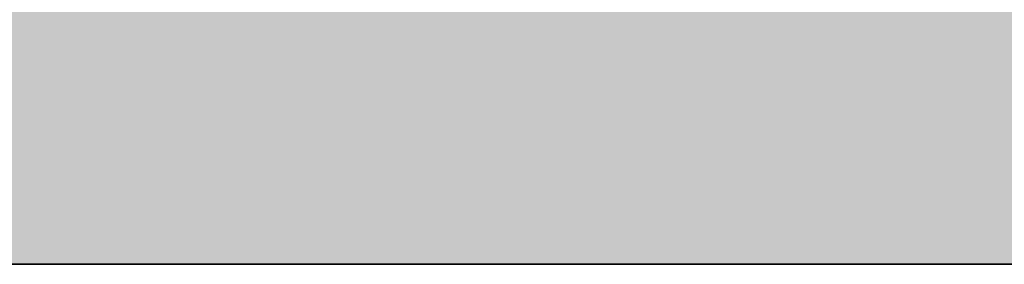
# Model space of a CAD drawing. Units: inches. Extents: x 2083 to 3317, y 1141 to 2115.
# Tile 147 of 256: x 3126.92826 to 3126.94671, y 1263.26136 to 1263.26594. Entities that reach past the tile are written whole.
import ezdxf

# ---------------------------------------------------------------- set-up
doc = ezdxf.new("R2010")
doc.units = ezdxf.units.IN
doc.layers.add('A-ANNO-DIMS', color=2, linetype='Continuous', lineweight=18)
doc.layers.add('A-WALL', color=7, linetype='Continuous', lineweight=35)
doc.layers.add('A-WALL-PATT', color=251, linetype='Continuous', lineweight=13, true_color=0x636466)
doc.styles.get("Standard").update_dxf_attribs({"font": 'arial.ttf'})
doc.dimstyles.new('ISO-25', dxfattribs={"dimtxt": 12, "dimasz": 12, "dimexe": 1.25, "dimexo": 0.625, "dimtad": 1, "dimlunit": 3, "dimtxsty": 'Standard', "dimcen": 2.5, "dimadec": 0, "dimazin": 0, "dimtfac": 1, "dimtmove": 0, "dimatfit": 3, "dimfxl": 1, "dimarcsym": 0})

# ---------------------------------------------------------------- blocks, each defined once
blk = doc.blocks.new('*D10')
at = {"layer": 'A-ANNO-DIMS', "color": 0, "lineweight": -2, "transparency": 16777216}
for p, q in [((2862.959783, 1262.63636), (2862.959783, 1201.38445)), ((3126.959783, 1262.63636), (3126.959783, 1201.38445)), ((2874.959783, 1202.63445), (3114.959783, 1202.63445))]:
    blk.add_line(p, q, dxfattribs=at)
at = {"layer": 'A-ANNO-DIMS', "color": 0, "transparency": 16777216}
for points in [[(2874.959783, 1204.63445), (2874.959783, 1200.63445), (2862.959783, 1202.63445)], [(3114.959783, 1204.63445), (3114.959783, 1200.63445), (3126.959783, 1202.63445)]]:
    blk.add_solid(points, dxfattribs=at)
at = {"layer": 'Defpoints', "color": 0, "transparency": 16777216}
for p in [(2862.959783, 1263.26136), (3126.959783, 1263.26136), (3126.959783, 1202.63445)]:
    blk.add_point(p, dxfattribs=at)
at = {"layer": 'A-ANNO-DIMS', "color": 0, "transparency": 16777216, "insert": (2994.959783, 1209.284006), "char_height": 12, "attachment_point": 5}
blk.add_mtext("22'", dxfattribs=at)
blk = doc.blocks.new('*D26')
at = {"layer": 'A-ANNO-DIMS', "color": 0, "lineweight": -2, "transparency": 16777216}
for p, q in [((3088.985844, 1274.915092), (3088.985844, 1270.951963)), ((3111.240037, 1274.915092), (3111.240037, 1270.951963)), ((3076.985844, 1272.201963), (2840.262447, 1272.201963)), ((3111.240037, 1272.201963), (3088.985844, 1272.201963)), ((3123.240037, 1272.201963), (3135.240037, 1272.201963))]:
    blk.add_line(p, q, dxfattribs=at)
at = {"layer": 'A-ANNO-DIMS', "color": 0, "transparency": 16777216}
for points in [[(3076.985844, 1274.201963), (3076.985844, 1270.201963), (3088.985844, 1272.201963)], [(3123.240037, 1274.201963), (3123.240037, 1270.201963), (3111.240037, 1272.201963)]]:
    blk.add_solid(points, dxfattribs=at)
at = {"layer": 'Defpoints', "color": 0, "transparency": 16777216}
for p in [(3088.985844, 1275.540092), (3111.240037, 1275.540092), (3088.985844, 1272.201963)]:
    blk.add_point(p, dxfattribs=at)
at = {"layer": 'A-ANNO-DIMS', "color": 0, "transparency": 16777216, "insert": (2952.624146, 1279.031602), "char_height": 12, "attachment_point": 5}
blk.add_mtext('NIGHTSTAND 1\'-10 1/2" TYP.', dxfattribs=at)
blk = doc.blocks.new('*D27')
at = {"layer": 'A-ANNO-DIMS', "color": 0, "lineweight": -2, "transparency": 16777216}
for p, q in [((3114.578165, 1309.794285), (3114.578165, 1321.794285)), ((3111.865037, 1297.794285), (3115.828165, 1297.794285)), ((3114.578165, 1297.794285), (3114.578165, 1275.540092)), ((3111.865037, 1275.540092), (3115.828165, 1275.540092)), ((3114.578165, 1263.540092), (3114.578165, 1140.988591))]:
    blk.add_line(p, q, dxfattribs=at)
at = {"layer": 'A-ANNO-DIMS', "color": 0, "transparency": 16777216}
for points in [[(3112.578165, 1309.794285), (3116.578165, 1309.794285), (3114.578165, 1297.794285)], [(3112.578165, 1263.540092), (3116.578165, 1263.540092), (3114.578165, 1275.540092)]]:
    blk.add_solid(points, dxfattribs=at)
at = {"layer": 'Defpoints', "color": 0, "transparency": 16777216}
for p in [(3111.240037, 1297.794285), (3111.240037, 1275.540092), (3114.578165, 1275.540092)]:
    blk.add_point(p, dxfattribs=at)
at = {"layer": 'A-ANNO-DIMS', "color": 0, "transparency": 16777216, "insert": (3107.748527, 1196.264342), "char_height": 12, "attachment_point": 5, "rotation": 90}
blk.add_mtext('1\'-10 1/2" TYP.', dxfattribs=at)

msp = doc.modelspace()

# ---------------------------------------------------------------- hatches: boundary and pattern name
at = {"layer": 'A-WALL-PATT'}
h = msp.add_hatch(color=256, dxfattribs=at)
h.dxf.hatch_style = 1
h.paths.add_polyline_path([(3126.959783, 2020.76136), (2748.959783, 2020.76136), (2604.959783, 2020.76136), (2226.959783, 2020.76136), (2226.959783, 1702.76136), (2466.959783, 1702.76136), (2466.959783, 1582.76136), (2418.959783, 1582.76136), (2418.959783, 1477.76136), (2226.959783, 1477.76136), (2226.959783, 1263.26136), (2544.959783, 1263.26136), (2544.959783, 1411.76136), (2604.959783, 1411.76136), (2685.959783, 1411.76136), (2685.959783, 1420.76136), (2604.959783, 1420.76136), (2604.959783, 1573.76136), (2604.959783, 1702.76136), (2604.959783, 2011.76136), (2748.959783, 2011.76136), (2748.959783, 1702.76136), (2862.959783, 1702.76136), (2862.959783, 1621.76136), (2871.959783, 1621.76136), (2871.959783, 1702.76136), (2883.959783, 1702.76136), (2883.959783, 1706.939459, -0.026459), (2883.959783, 1711.76136), (2757.959783, 1711.76136), (2757.959783, 1807.76136), (2787.959783, 1807.76136), (2787.959783, 1812.26136), (2757.959783, 1812.26136), (2757.959783, 2011.76136), (2877.959783, 2011.76136), (2877.959783, 1812.26136), (2847.959783, 1812.26136), (2847.959783, 1807.76136), (2889.835742, 1807.76136), (2889.835742, 1812.26136), (2882.459783, 1812.26136), (2882.459783, 2011.76136), (3117.959783, 2011.76136), (3117.959783, 1812.26136), (2937.835742, 1812.26136), (2937.835742, 1807.76136), (2995.709783, 1807.76136), (2995.709783, 1796.117666), (3000.209783, 1796.117666), (3000.209783, 1807.76136), (3117.959783, 1807.76136), (3117.959783, 1711.76136), (3000.209783, 1711.76136), (3000.209783, 1760.117666), (2998.572705, 1760.117666, -0.020711), (2995.709783, 1760.117666), (2995.709783, 1711.76136), (2931.959783, 1711.76136), (2931.959783, 1702.76136), (3126.959783, 1702.76136)])
h.paths.add_polyline_path([(2471.459783, 2011.76136), (2471.459783, 1810.01136), (2462.716936, 1810.01136), (2462.716936, 1805.51136), (2505.959783, 1805.51136), (2505.959783, 1810.01136), (2475.959783, 1810.01136), (2475.959783, 2011.76136), (2595.959783, 2011.76136), (2595.959783, 1810.01136), (2565.959783, 1810.01136), (2565.959783, 1805.51136), (2595.959783, 1805.51136), (2595.959783, 1711.76136), (2235.959783, 1711.76136), (2235.959783, 1805.51136), (2353.709783, 1805.51136), (2353.709783, 1796.054162), (2358.209783, 1796.054162), (2358.209783, 1805.51136), (2414.716936, 1805.51136), (2414.716936, 1810.01136), (2235.959783, 1810.01136), (2235.959783, 2011.76136)], flags=16)
h.paths.add_polyline_path([(2270.204734, 1994.610008), (2270.204734, 1970.610008), (2246.204734, 1970.610008), (2246.204734, 1994.610008)], flags=0)
edge = h.paths.add_edge_path(flags=0)
edge.add_ellipse((2332.027391, 1899.798176), major_axis=(-3.042994, 3.042994), ratio=0.16825245, start_angle=-161.332166, end_angle=-156.307114, ccw=False)
edge.add_ellipse((2333.082037, 1898.74353), major_axis=(-1.054646, 1.054646), ratio=0.4535321, start_angle=-123.371019, end_angle=-94.159107)
edge = h.paths.add_edge_path(flags=0)
edge.add_ellipse((2332.027391, 1968.87629), major_axis=(3.042994, 3.042994), ratio=0.16825245, start_angle=18.667834, end_angle=23.692886)
edge.add_spline(control_points=[(2332.925596, 1970.691105), (2332.226768, 1970.3361), (2330.893709, 1969.658905), (2328.41308, 1970.932138), (2327.203934, 1967.748712), (2324.709596, 1969.955589), (2322.532822, 1967.012354), (2320.012846, 1971.295812), (2317.680308, 1968.157845), (2316.040526, 1967.102047), (2315.426904, 1966.809602)], knot_values=[0, 0, 0, 0, 2.267059, 4.324559, 6.685584, 8.878641, 11.121502, 14.300359, 17.755284, 19.732645, 19.732645, 19.732645, 19.732645], degree=3, periodic=0)
edge.add_ellipse((2332.027391, 1968.87629), major_axis=(3.042994, 3.042994), ratio=0.16825245, start_angle=18.667834, end_angle=23.692886, ccw=False)
edge.add_ellipse((2333.082037, 1969.930936), major_axis=(1.054646, 1.054646), ratio=0.4535321, start_angle=56.628981, end_angle=85.840893, ccw=False)
edge = h.paths.add_edge_path(flags=0)
edge.add_spline(control_points=[(2296.428287, 1967.987908), (2293.627804, 1965.336314), (2287.703624, 1959.727094), (2299.74386, 1949.995699), (2294.532591, 1935.668528), (2290.573228, 1920.603512), (2293.394124, 1909.973691), (2296.185407, 1904.966543)], knot_values=[0.099185, 0.099185, 0.099185, 0.099185, 0.345301, 0.619822, 0.982653, 1.386093, 1.810555, 1.810555, 1.810555, 1.810555], degree=3, periodic=0)
edge.add_spline(control_points=[(2296.185407, 1904.966543), (2297.383582, 1902.6193), (2298.000969, 1901.949312), (2298.55297, 1901.468155)], knot_values=[0.006246, 0.006246, 0.006246, 0.006246, 0.055476, 0.055476, 0.055476, 0.055476], degree=3, periodic=0)
edge.add_spline(control_points=[(2298.55297, 1901.468155), (2297.258612, 1900.923224), (2295.225294, 1900.232126), (2293.060229, 1900.614205), (2292.101423, 1900.788415), (2292.089578, 1900.790568)], knot_values=[0.312835, 0.312835, 0.312835, 0.312835, 0.40178, 0.474987, 0.475903, 0.475903, 0.475903, 0.475903], degree=3, periodic=0)
edge.add_arc((2292.793646, 1904.664109), 3.937008, 215.420897, 259.698179, ccw=False)
edge.add_spline(control_points=[(2289.585314, 1902.382304), (2289.476652, 1902.535087), (2289.36848, 1902.688035), (2289.260865, 1902.84117)], knot_values=[0.102872, 0.102872, 0.102872, 0.102872, 0.116896, 0.116896, 0.116896, 0.116896], degree=3, periodic=0)
edge.add_spline(control_points=[(2289.260865, 1902.84117), (2288.686604, 1902.550192), (2287.640048, 1902.019902), (2285.881337, 1901.873954), (2283.852972, 1901.504352), (2281.719987, 1899.710538), (2278.466991, 1899.492942), (2276.157136, 1901.883202), (2272.258953, 1899.804071), (2267.777605, 1901.843183), (2262.243882, 1900.184033), (2257.414927, 1901.782061), (2254.318374, 1900.72612), (2253.178285, 1900.337343)], knot_values=[0, 0, 0, 0, 1.907977, 3.477176, 5.261074, 7.972851, 11.680248, 13.717921, 16.939592, 22.789562, 27.502503, 33.595215, 37.145618, 37.145618, 37.145618, 37.145618], degree=3, periodic=0)
edge.add_line((2253.178285, 1900.337343), (2250.24424, 1902.84117))
edge.add_line((2250.24424, 1902.84117), (2250.24424, 1965.833296))
edge.add_line((2250.24424, 1965.833296), (2253.178285, 1968.337123))
edge.add_spline(control_points=[(2253.178285, 1968.337123), (2254.318374, 1967.948346), (2257.414927, 1966.892405), (2262.243882, 1968.490433), (2267.777605, 1966.831283), (2271.52673, 1968.537217), (2273.875914, 1967.828289), (2274.206701, 1967.727642)], knot_values=[0, 0, 0, 0, 0.09018, 0.244935, 0.364644, 0.513233, 0.537855, 0.537855, 0.537855, 0.537855], degree=3, periodic=0)
edge.add_arc((2274.352887, 1963.793349), 3.937008, 72.051134, 92.127949, ccw=False)
edge.add_arc((2281.296933, 1985.230003), 18.596298, 252.0511336, 288.5657217)
edge.add_arc((2292.316717, 1956.02888), 12.646081, 71.0267879, 113.7782184, ccw=False)
edge = h.paths.add_edge_path(flags=0)
edge.add_spline(control_points=[(2274.899415, 1951.856195), (2275.066156, 1951.616592), (2275.232687, 1951.376588), (2275.397987, 1951.135855)], knot_values=[1.409916, 1.409916, 1.409916, 1.409916, 1.43159, 1.43159, 1.43159, 1.43159], degree=3, periodic=0)
edge.add_spline(control_points=[(2275.397987, 1951.135855), (2275.792106, 1950.561885), (2276.179231, 1949.983774), (2276.545546, 1949.397103)], knot_values=[1.358238, 1.358238, 1.358238, 1.358238, 1.409916, 1.409916, 1.409916, 1.409916], degree=3, periodic=0)
edge.add_line((2276.545546, 1949.397103), (2277.437289, 1947.862185))
edge.add_spline(control_points=[(2277.437289, 1947.862185), (2276.303834, 1945.673115), (2274.639698, 1942.426882), (2274.631615, 1938.0939), (2272.799124, 1930.85155), (2274.356426, 1943.897046), (2275.947681, 1947.923356), (2276.545546, 1949.397103)], knot_values=[0.005632, 0.005632, 0.005632, 0.005632, 0.186014, 0.266002, 0.357087, 0.59639, 0.739732, 0.739732, 0.739732, 0.739732], degree=3, periodic=0)
edge.add_spline(control_points=[(2276.545546, 1949.397103), (2276.179231, 1949.983774), (2275.792106, 1950.561885), (2275.397987, 1951.135855)], knot_values=[1.358238, 1.358238, 1.358238, 1.358238, 1.409916, 1.409916, 1.409916, 1.409916], degree=3, periodic=0)
edge.add_spline(control_points=[(2275.397987, 1951.135855), (2274.9425, 1950.080452), (2274.20776, 1948.025272), (2273.934602, 1944.851477), (2272.468534, 1937.627489), (2273.466216, 1945.696466), (2274.700615, 1951.059472), (2274.899415, 1951.856195)], knot_values=[0.104364, 0.104364, 0.104364, 0.104364, 0.189636, 0.269624, 0.36071, 0.600013, 0.644622, 0.644622, 0.644622, 0.644622], degree=3, periodic=0)
h.paths.add_polyline_path([(2269.167514, 1963.127573, -0.357527), (2268.170633, 1960.97637, -0.092561), (2268.170633, 1939.436325, -0.357527), (2269.167514, 1937.285122, -0.357527), (2267.01631, 1938.282002, -0.164785), (2254.685581, 1938.282002, -0.357527), (2252.534378, 1937.285122, -0.357527), (2253.531259, 1939.436325, -0.092561), (2253.531259, 1960.97637, -0.357527), (2252.534378, 1963.127573, -0.357527), (2254.685581, 1962.130692, -0.164785), (2267.01631, 1962.130692, -0.357527)], flags=0)
h.paths.add_polyline_path([(2248.874068, 1967.8018), (2248.874068, 1957.02771), (2249.457783, 1957.02771), (2249.457783, 1911.646756), (2248.874068, 1911.646756), (2248.874068, 1900.872666), (2246.511863, 1900.872666, 0.197327), (2244.149658, 1902.456873), (2244.149658, 1966.217592, 0.197327), (2246.511863, 1967.8018)], flags=0)
h.paths.add_polyline_path([(2269.167514, 1931.389344, -0.357527), (2268.170633, 1929.238141, -0.092561), (2268.170633, 1907.698096, -0.357527), (2269.167514, 1905.546893, -0.357527), (2267.01631, 1906.543774, -0.164785), (2254.685581, 1906.543774, -0.357527), (2252.534378, 1905.546893, -0.357527), (2253.531259, 1907.698096, -0.092561), (2253.531259, 1929.238141, -0.357527), (2252.534378, 1931.389344, -0.357527), (2254.685581, 1930.392463, -0.164785), (2267.01631, 1930.392463, -0.357527)], flags=0)
edge = h.paths.add_edge_path(flags=0)
edge.add_spline(control_points=[(2276.196858, 1906.723702), (2276.168144, 1909.028928), (2276.114049, 1913.371852), (2270.598417, 1924.924978), (2273.905175, 1919.012779), (2275.921711, 1916.262063), (2275.47457, 1912.402149), (2277.257874, 1910.380621), (2276.696044, 1908.225036), (2276.646218, 1906.813023), (2276.617825, 1906.008407)], knot_values=[0, 0, 0, 0, 8.61026, 16.221274, 18.843057, 23.804898, 27.440828, 29.356102, 31.203478, 33.650687, 33.650687, 33.650687, 33.650687], degree=3, periodic=0)
edge.add_spline(control_points=[(2276.617825, 1906.008407), (2276.623313, 1905.624144), (2276.497738, 1904.628661), (2275.441779, 1903.854725), (2274.937314, 1903.08045), (2274.85908, 1902.84117)], knot_values=[0.156488, 0.156488, 0.156488, 0.156488, 0.184398, 0.231376, 0.250598, 0.250598, 0.250598, 0.250598], degree=3, periodic=0)
edge.add_line((2274.85908, 1902.84117), (2276.50598, 1902.84117))
edge.add_spline(control_points=[(2276.50598, 1902.84117), (2276.788308, 1903.08494), (2277.665071, 1904.125196), (2278.249538, 1904.340738), (2277.653872, 1908.527387), (2278.15567, 1906.227808), (2278.100464, 1905.285948), (2278.846675, 1904.069005), (2277.856785, 1903.414948), (2277.874191, 1902.99105), (2277.903562, 1902.84117)], knot_values=[0.059574, 0.059574, 0.059574, 0.059574, 0.080753, 0.103741, 0.16972, 0.176036, 0.207137, 0.240474, 0.262341, 0.27366, 0.27366, 0.27366, 0.27366], degree=3, periodic=0)
edge.add_line((2277.903562, 1902.84117), (2280.029825, 1902.84117))
edge.add_spline(control_points=[(2280.029825, 1902.84117), (2279.888221, 1903.088398), (2279.499257, 1903.981551), (2280.152284, 1905.939349), (2278.103615, 1909.657757), (2279.762395, 1907.185285), (2280.3279, 1904.874861), (2280.485109, 1903.48959), (2281.463269, 1903.249432), (2281.758343, 1902.936497), (2281.834036, 1902.84117)], knot_values=[0.013856, 0.013856, 0.013856, 0.013856, 0.034874, 0.088867, 0.107879, 0.126738, 0.158714, 0.193757, 0.217487, 0.226722, 0.226722, 0.226722, 0.226722], degree=3, periodic=0)
edge.add_spline(control_points=[(2281.834036, 1902.84117), (2281.787535, 1902.826703), (2281.647022, 1902.782988), (2281.395527, 1902.85949), (2281.088077, 1902.985242), (2280.720683, 1903.060902), (2280.333451, 1903.025726), (2280.124767, 1902.898879), (2280.029825, 1902.84117)], knot_values=[0, 0, 0, 0, 0.14413, 0.435517, 0.749276, 1.153046, 1.548371, 1.878348, 1.878348, 1.878348, 1.878348], degree=3, periodic=0)
edge.add_line((2280.029825, 1902.84117), (2277.903562, 1902.84117))
edge.add_spline(control_points=[(2277.903562, 1902.84117), (2277.892855, 1902.795855), (2277.865396, 1902.679637), (2277.607479, 1902.687483), (2277.27405, 1902.8007), (2276.837921, 1902.619775), (2276.583807, 1902.789261), (2276.50598, 1902.84117)], knot_values=[0, 0, 0, 0, 0.127189, 0.326199, 0.628009, 1.24357, 1.515331, 1.515331, 1.515331, 1.515331], degree=3, periodic=0)
edge.add_line((2276.50598, 1902.84117), (2274.85908, 1902.84117))
edge.add_spline(control_points=[(2274.85908, 1902.84117), (2274.814437, 1902.898587), (2274.72513, 1903.013446), (2274.493477, 1903.118968), (2274.244285, 1902.960539), (2273.937121, 1903.184942), (2273.614039, 1902.983143), (2273.408316, 1902.883045), (2273.322254, 1902.84117)], knot_values=[0, 0, 0, 0, 0.21843, 0.436957, 0.687977, 0.990379, 1.398396, 1.69185, 1.69185, 1.69185, 1.69185], degree=3, periodic=0)
edge.add_spline(control_points=[(2273.322254, 1902.84117), (2273.61674, 1903.445692), (2274.273998, 1904.538253), (2276.027239, 1904.573702), (2276.206963, 1906.583637), (2276.196858, 1906.723702)], knot_values=[0.012227, 0.012227, 0.012227, 0.012227, 0.059472, 0.106218, 0.134458, 0.134458, 0.134458, 0.134458], degree=3, periodic=0)
h.paths.add_polyline_path([(2270.776054, 1897.789828), (2270.776054, 1873.789828), (2246.776054, 1873.789828), (2246.776054, 1897.789828)], flags=0)
h.paths.add_polyline_path([(2353.709783, 1760.005059), (2353.709783, 1760.054162), (2358.209783, 1760.054162, -0.033729)], flags=0)
h.paths.add_polyline_path([(2321.819119, 1737.529186), (2341.995327, 1737.529186, -0.414214), (2343.203273, 1736.321241), (2343.203273, 1721.020596, -0.414214), (2341.995327, 1719.812651), (2321.819119, 1719.812651, -0.414214), (2320.611173, 1721.020596), (2320.611173, 1736.321241, -0.414214)], flags=0)
h.paths.add_polyline_path([(2324.23501, 1736.321241), (2339.579436, 1736.321241, -0.414214), (2341.995327, 1733.905349), (2341.995327, 1725.44973, -0.414214), (2339.579436, 1723.033839), (2333.680588, 1723.033839), (2333.845317, 1722.045467, -0.870646), (2335.425399, 1721.825893, -0.767327), (2333.922694, 1721.423245), (2331.291024, 1721.423245, -0.767327), (2329.788319, 1721.825893, -0.870646), (2331.368401, 1722.045467), (2331.53313, 1723.033839), (2324.23501, 1723.033839, -0.414214), (2321.819119, 1725.44973), (2321.819119, 1733.905349, -0.414214)], flags=0)
h.paths.add_polyline_path([(2570.483789, 1928.615444), (2589.683789, 1928.615444), (2590.168829, 1928.615444), (2590.168829, 1904.993397), (2570.483789, 1904.993397)], flags=0)
h.paths.add_polyline_path([(2574.447324, 1927.263822, -1), (2572.828836, 1927.263822, -1)], flags=0)
h.paths.add_polyline_path([(2573.089867, 1926.940877), (2573.925032, 1927.776042), (2574.147743, 1927.553332), (2573.312577, 1926.718166)], flags=0)
h.paths.add_polyline_path([(2578.779065, 1919.729618, -1), (2571.591663, 1919.729618, -1)], flags=0)
h.paths.add_polyline_path([(2578.385364, 1919.729618, -1), (2571.985364, 1919.729618, -1)], flags=0)
h.paths.add_polyline_path([(2331.595764, 1729.476216, -1), (2333.617954, 1729.476216, -1)], flags=0)
h.paths.add_polyline_path([(2578.034228, 1927.263822, -1), (2576.41574, 1927.263822, -1)], flags=0)
h.paths.add_polyline_path([(2576.688851, 1927.531089), (2576.911562, 1927.753799), (2577.746728, 1926.918634), (2577.524017, 1926.695923)], flags=0)
h.paths.add_polyline_path([(2578.139065, 1909.859539, -1), (2572.231663, 1909.859539, -1)], flags=0)
h.paths.add_polyline_path([(2577.745364, 1909.859539, -1), (2572.625364, 1909.859539, -1)], flags=0)
h.paths.add_polyline_path([(2583.797718, 1927.263822, -1), (2582.179229, 1927.263822, -1)], flags=0)
h.paths.add_polyline_path([(2582.718649, 1927.753799), (2583.553814, 1926.918634), (2583.331103, 1926.695923), (2582.495938, 1927.531089)], flags=0)
h.paths.add_polyline_path([(2582.495938, 1927.531089), (2582.718649, 1927.753799), (2583.553814, 1926.918634), (2583.331103, 1926.695923)], flags=0)
h.paths.add_polyline_path([(2587.739065, 1920.529618, -1), (2581.831663, 1920.529618, -1)], flags=0)
h.paths.add_polyline_path([(2587.345364, 1920.529618, -1), (2582.225364, 1920.529618, -1)], flags=0)
h.paths.add_polyline_path([(2587.384622, 1927.263822, -1), (2585.766133, 1927.263822, -1)], flags=0)
h.paths.add_polyline_path([(2586.081993, 1926.980247), (2586.917158, 1927.815412), (2587.139869, 1927.592702), (2586.304703, 1926.757536)], flags=0)
h.paths.add_polyline_path([(2588.379065, 1910.659539, -1), (2581.191663, 1910.659539, -1)], flags=0)
h.paths.add_polyline_path([(2587.985364, 1910.659539, -1), (2581.585364, 1910.659539, -1)], flags=0)
h.paths.add_polyline_path([(2417.167729, 1729.477895), (2437.343937, 1729.477895, -0.414214), (2438.551883, 1728.26995), (2438.551883, 1712.969306, -0.414214), (2437.343937, 1711.76136), (2417.167729, 1711.76136, -0.414214), (2415.959783, 1712.969306), (2415.959783, 1728.26995, -0.414214)], flags=0)
h.paths.add_polyline_path([(2419.58362, 1728.26995), (2434.928046, 1728.26995, -0.414214), (2437.343937, 1725.854059), (2437.343937, 1717.39844, -0.414214), (2434.928046, 1714.982548), (2429.029199, 1714.982548), (2429.193927, 1713.994176, -0.870646), (2430.774009, 1713.774603, -0.767327), (2429.271304, 1713.371954), (2426.639634, 1713.371954, -0.767327), (2425.136929, 1713.774603, -0.870646), (2426.717011, 1713.994176), (2426.88174, 1714.982548), (2419.58362, 1714.982548, -0.414214), (2417.167729, 1717.39844), (2417.167729, 1725.854059, -0.414214)], flags=0)
h.paths.add_polyline_path([(2419.58362, 1728.26995), (2434.928046, 1728.26995, -0.414214), (2437.343937, 1725.854059), (2437.343937, 1717.39844, -0.414214), (2434.928046, 1714.982548), (2429.029199, 1714.982548), (2428.358118, 1719.009034), (2427.552821, 1719.009034), (2426.88174, 1714.982548), (2419.58362, 1714.982548, -0.414214), (2417.167729, 1717.39844), (2417.167729, 1725.854059, -0.414214)], flags=0)
h.paths.add_polyline_path([(2426.944374, 1721.424925, -1), (2428.966564, 1721.424925, -1)], flags=0)
h.paths.add_polyline_path([(2475.959783, 1702.76136), (2595.959783, 1702.76136), (2595.959783, 1582.76136), (2475.959783, 1582.76136)], flags=16)
h.paths.add_polyline_path([(2427.959783, 1573.76136), (2595.959783, 1573.76136), (2595.959783, 1468.76136), (2595.959783, 1420.76136), (2384.459783, 1420.76136), (2384.459783, 1468.76136), (2427.959783, 1468.76136)], flags=16)
h.paths.add_polyline_path([(2379.959783, 1468.76136), (2379.959783, 1420.76136), (2235.959783, 1420.76136), (2235.959783, 1468.76136)], flags=16)
h.paths.add_polyline_path([(2317.815996, 1466.695767), (2337.992205, 1466.695767, -0.414214), (2339.20015, 1465.487821), (2339.20015, 1450.187177, -0.414214), (2337.992205, 1448.979232), (2317.815996, 1448.979232, -0.414214), (2316.608051, 1450.187177), (2316.608051, 1465.487821, -0.414214)], flags=0)
h.paths.add_polyline_path([(2320.231887, 1465.487821), (2335.576313, 1465.487821, -0.414214), (2337.992205, 1463.07193), (2337.992205, 1454.616311, -0.414214), (2335.576313, 1452.20042), (2329.677466, 1452.20042), (2329.842195, 1451.212047, -0.870646), (2331.422276, 1450.992474, -0.767327), (2329.919571, 1450.589826), (2327.287902, 1450.589826, -0.767327), (2325.785197, 1450.992474, -0.870646), (2327.365278, 1451.212047), (2327.530007, 1452.20042), (2320.231887, 1452.20042, -0.414214), (2317.815996, 1454.616311), (2317.815996, 1463.07193, -0.414214)], flags=0)
h.paths.add_polyline_path([(2320.231887, 1465.487821), (2335.576313, 1465.487821, -0.414214), (2337.992205, 1463.07193), (2337.992205, 1454.616311, -0.414214), (2335.576313, 1452.20042), (2329.677466, 1452.20042), (2329.006385, 1456.226905), (2328.201088, 1456.226905), (2327.530007, 1452.20042), (2320.231887, 1452.20042, -0.414214), (2317.815996, 1454.616311), (2317.815996, 1463.07193, -0.414214)], flags=0)
h.paths.add_polyline_path([(2327.592641, 1458.642796, -1), (2329.614832, 1458.642796, -1)], flags=0)
h.paths.add_polyline_path([(2244.411744, 1433.340453), (2241.920945, 1433.340453, -0.414214), (2240.017856, 1435.243542), (2240.017856, 1440.952808, -0.414211), (2241.920925, 1442.855897), (2244.411744, 1442.855897, -1.976472)], flags=0)
h.paths.add_polyline_path([(2245.356888, 1434.397536, -0.414214), (2245.356888, 1441.798814, -2.144098)], flags=0)
h.paths.add_polyline_path([(2535.959783, 1416.26136), (2535.959783, 1272.26136), (2235.959783, 1272.26136), (2235.959783, 1416.26136)], flags=16)
h.paths.add_polyline_path([(2260.119561, 1384.292841), (2260.119561, 1362.038649), (2237.865369, 1362.038649), (2237.865369, 1384.292841)], flags=0)
edge = h.paths.add_edge_path(flags=0)
edge.add_line((2318.251847, 1362.093298), (2318.145797, 1362.000973))
edge.add_ellipse((2317.445116, 1360.431044), major_axis=(2.82164, 2.82164), ratio=0.16825245, start_angle=18.667834, end_angle=20.948127, ccw=False)
edge.add_ellipse((2318.423045, 1361.408974), major_axis=(0.977929, 0.977929), ratio=0.4535321, start_angle=56.628981, end_angle=70.226201, ccw=False)
edge = h.paths.add_edge_path(flags=0)
edge.add_line((2319.10737, 1295.571078), (2319.015044, 1295.677128))
edge.add_ellipse((2317.445116, 1296.377809), major_axis=(-2.82164, 2.82164), ratio=0.16825245, start_angle=-161.332166, end_angle=-159.051873, ccw=False)
edge.add_ellipse((2318.423045, 1295.39988), major_axis=(-0.977929, 0.977929), ratio=0.4535321, start_angle=-123.371019, end_angle=-109.773799)
edge = h.paths.add_edge_path(flags=0)
edge.add_spline(control_points=[(2284.210349, 1301.170219), (2284.580688, 1300.444719), (2284.891189, 1299.892024), (2285.159553, 1299.461018)], knot_values=[0.039066, 0.039066, 0.039066, 0.039066, 0.055476, 0.055476, 0.055476, 0.055476], degree=3, periodic=0)
edge.add_line((2285.159553, 1299.461018), (2284.210349, 1301.170219))
edge = h.paths.add_edge_path(flags=0)
edge.add_line((2280.412458, 1297.298013), (2283.369991, 1297.036122))
edge.add_line((2283.369991, 1297.036122), (2286.40569, 1297.92631))
edge.add_spline(control_points=[(2286.40569, 1297.92631), (2285.305487, 1297.463119), (2284.344777, 1297.129151), (2283.369991, 1297.036122)], knot_values=[0.394369, 0.394369, 0.394369, 0.394369, 0.475903, 0.475903, 0.475903, 0.475903], degree=3, periodic=0)
edge.add_spline(control_points=[(2283.369991, 1297.036122), (2283.28139, 1297.027666), (2282.316289, 1296.957336), (2281.312502, 1297.134479), (2280.423441, 1297.296016), (2280.412458, 1297.298013)], knot_values=[0.312835, 0.312835, 0.312835, 0.312835, 0.320246, 0.393453, 0.394369, 0.394369, 0.394369, 0.394369], degree=3, periodic=0)
edge = h.paths.add_edge_path(flags=0)
edge.add_line((2284.435561, 1359.607285), (2280.446291, 1355.328047))
edge.add_line((2280.446291, 1355.328047), (2279.579987, 1351.017754))
edge.add_line((2279.579987, 1351.017754), (2282.412974, 1346.580433))
edge.add_spline(control_points=[(2282.412974, 1346.580433), (2283.153331, 1345.589236), (2284.252896, 1344.028897), (2284.801037, 1342.387167), (2284.935162, 1341.805544)], knot_values=[1.240098, 1.240098, 1.240098, 1.240098, 1.332892, 1.382712, 1.382712, 1.382712, 1.382712], degree=3, periodic=0)
edge.add_spline(control_points=[(2284.935162, 1341.805544), (2285.319108, 1340.1406), (2285.233029, 1338.409204), (2284.909938, 1336.654122)], knot_values=[1.097484, 1.097484, 1.097484, 1.097484, 1.240098, 1.240098, 1.240098, 1.240098], degree=3, periodic=0)
edge.add_spline(control_points=[(2284.909938, 1336.654122), (2284.586848, 1334.89904), (2284.026745, 1333.120272), (2283.462644, 1331.360585)], knot_values=[0.95487, 0.95487, 0.95487, 0.95487, 1.097484, 1.097484, 1.097484, 1.097484], degree=3, periodic=0)
edge.add_line((2283.462644, 1331.360585), (2281.890376, 1326.153357))
edge.add_line((2281.890376, 1326.153357), (2280.756259, 1321.056089))
edge.add_line((2280.756259, 1321.056089), (2280.299205, 1316.001977))
edge.add_line((2280.299205, 1316.001977), (2280.715933, 1310.950068))
edge.add_line((2280.715933, 1310.950068), (2282.028094, 1305.972137))
edge.add_line((2282.028094, 1305.972137), (2284.210349, 1301.170219))
edge.add_spline(control_points=[(2284.210349, 1301.170219), (2283.340731, 1302.730185), (2282.611904, 1304.336493), (2282.028094, 1305.972137)], knot_values=[0.099185, 0.099185, 0.099185, 0.099185, 0.241799, 0.241799, 0.241799, 0.241799], degree=3, periodic=0)
edge.add_spline(control_points=[(2282.028094, 1305.972137), (2281.444283, 1307.60778), (2281.005489, 1309.272759), (2280.715933, 1310.950068)], knot_values=[0.241799, 0.241799, 0.241799, 0.241799, 0.384413, 0.384413, 0.384413, 0.384413], degree=3, periodic=0)
edge.add_spline(control_points=[(2280.715933, 1310.950068), (2280.433241, 1312.587613), (2280.289386, 1314.276959), (2280.298894, 1315.962032), (2280.299205, 1316.001977)], knot_values=[0.384413, 0.384413, 0.384413, 0.384413, 0.523647, 0.527028, 0.527028, 0.527028, 0.527028], degree=3, periodic=0)
edge.add_spline(control_points=[(2280.299205, 1316.001977), (2280.312326, 1317.686955), (2280.477871, 1319.367926), (2280.756259, 1321.056089)], knot_values=[0.527028, 0.527028, 0.527028, 0.527028, 0.669642, 0.669642, 0.669642, 0.669642], degree=3, periodic=0)
edge.add_spline(control_points=[(2280.756259, 1321.056089), (2281.034648, 1322.744252), (2281.42588, 1324.439608), (2281.890376, 1326.153357)], knot_values=[0.669642, 0.669642, 0.669642, 0.669642, 0.812256, 0.812256, 0.812256, 0.812256], degree=3, periodic=0)
edge.add_spline(control_points=[(2281.890376, 1326.153357), (2282.264383, 1327.533251), (2282.78787, 1329.26181), (2283.352751, 1331.01778), (2283.462644, 1331.360585)], knot_values=[0.812256, 0.812256, 0.812256, 0.812256, 0.927087, 0.95487, 0.95487, 0.95487, 0.95487], degree=3, periodic=0)
edge.add_line((2283.462644, 1331.360585), (2284.909938, 1336.654122))
edge.add_line((2284.909938, 1336.654122), (2284.935162, 1341.805544))
edge.add_line((2284.935162, 1341.805544), (2282.412974, 1346.580433))
edge.add_spline(control_points=[(2282.412974, 1346.580433), (2281.275127, 1348.103792), (2280.078447, 1349.570318), (2279.579987, 1351.017754)], knot_values=[1.382712, 1.382712, 1.382712, 1.382712, 1.525326, 1.525326, 1.525326, 1.525326], degree=3, periodic=0)
edge.add_spline(control_points=[(2279.579987, 1351.017754), (2279.443282, 1351.414721), (2279.136312, 1352.856922), (2279.73519, 1354.290385), (2280.446291, 1355.328047)], knot_values=[1.525326, 1.525326, 1.525326, 1.525326, 1.564439, 1.667941, 1.667941, 1.667941, 1.667941], degree=3, periodic=0)
edge.add_spline(control_points=[(2280.446291, 1355.328047), (2281.426113, 1356.757835), (2282.930837, 1358.18256), (2284.435561, 1359.607285)], knot_values=[1.667941, 1.667941, 1.667941, 1.667941, 1.810555, 1.810555, 1.810555, 1.810555], degree=3, periodic=0)
edge.add_arc((2280.623075, 1348.518181), 11.72618, 71.0267879, 113.7782184)
edge.add_arc((2270.404892, 1375.595156), 17.243567, 252.0511336, 288.5657217, ccw=False)
edge.add_arc((2263.965969, 1355.717847), 3.650622, 72.051134, 92.127949)
edge.add_arc((2263.965969, 1355.717847), 3.650622, 92.127949, 177.98513)
edge.add_spline(control_points=[(2260.317604, 1355.846199), (2260.260417, 1354.220668), (2260.551278, 1350.186547), (2262.999344, 1346.766251), (2264.472741, 1344.649024)], knot_values=[1.43159, 1.43159, 1.43159, 1.43159, 1.564144, 1.770695, 1.770695, 1.770695, 1.770695], degree=3, periodic=0)
edge.add_line((2264.472741, 1344.649024), (2264.93559, 1343.98253))
edge.add_spline(control_points=[(2263.801044, 1340.248105), (2263.843238, 1340.514088), (2264.067244, 1341.756465), (2264.512693, 1343.002453), (2264.935047, 1343.981083)], knot_values=[0.53657, 0.53657, 0.53657, 0.53657, 0.559349, 0.644622, 0.644622, 0.644622, 0.644622], degree=3, periodic=0)
edge.add_spline(control_points=[(2264.935047, 1343.981083), (2265.117771, 1343.714975), (2265.298875, 1343.447906), (2265.476756, 1343.179365)], knot_values=[1.384077, 1.384077, 1.384077, 1.384077, 1.409916, 1.409916, 1.409916, 1.409916], degree=3, periodic=0)
edge.add_spline(control_points=[(2265.476756, 1343.179365), (2265.654637, 1342.910823), (2265.829296, 1342.64081), (2265.99913, 1342.368812)], knot_values=[1.358238, 1.358238, 1.358238, 1.358238, 1.384077, 1.384077, 1.384077, 1.384077], degree=3, periodic=0)
edge.add_line((2265.99913, 1342.368812), (2266.826006, 1340.945547))
edge.add_spline(control_points=[(2266.826006, 1340.945547), (2268.894401, 1337.089691), (2271.398173, 1325.843001), (2270.516164, 1310.568557), (2275.919376, 1301.860609), (2277.789511, 1299.19945)], knot_values=[0.116896, 0.116896, 0.116896, 0.116896, 0.472987, 1.050969, 1.313793, 1.313793, 1.313793, 1.313793], degree=3, periodic=0)
edge.add_spline(control_points=[(2277.789511, 1299.19945), (2277.839405, 1299.128452), (2277.889428, 1299.057498), (2277.939572, 1298.986584)], knot_values=[0.109884, 0.109884, 0.109884, 0.109884, 0.116896, 0.116896, 0.116896, 0.116896], degree=3, periodic=0)
edge.add_line((2277.939572, 1298.986584), (2277.788849, 1299.199114))
edge.add_spline(control_points=[(2277.788849, 1299.199114), (2277.256582, 1298.929414), (2276.28635, 1298.437902), (2275.039352, 1298.334419), (2274.38333, 1298.238895), (2274.215254, 1298.209338)], knot_values=[33.12187, 33.12187, 33.12187, 33.12187, 35.029056, 36.598255, 37.144827, 37.144827, 37.144827, 37.144827], degree=3, periodic=0)
edge.add_line((2274.215254, 1298.209338), (2273.073147, 1297.892961))
edge.add_spline(control_points=[(2273.073147, 1297.892961), (2272.322936, 1297.579784), (2271.039151, 1296.510508), (2269.248395, 1296.226062), (2268.4231, 1296.374654)], knot_values=[26.532584, 26.532584, 26.532584, 26.532584, 29.198919, 31.839101, 31.839101, 31.839101, 31.839101], degree=3, periodic=0)
edge.add_line((2268.4231, 1296.374654), (2263.878501, 1297.457534))
edge.add_spline(control_points=[(2263.878501, 1297.457534), (2263.556077, 1297.359435), (2261.860306, 1296.838694), (2260.23878, 1297.282407), (2258.933454, 1297.516461)], knot_values=[15.919551, 15.919551, 15.919551, 15.919551, 16.939592, 21.226067, 21.226067, 21.226067, 21.226067], degree=3, periodic=0)
edge.add_line((2258.933454, 1297.516461), (2254.055233, 1297.32901))
edge.add_spline(control_points=[(2254.055233, 1297.32901), (2253.755525, 1297.295815), (2252.113683, 1297.165174), (2250.461869, 1297.544221), (2249.129686, 1297.667882)], knot_values=[5.306517, 5.306517, 5.306517, 5.306517, 6.276435, 10.613034, 10.613034, 10.613034, 10.613034], degree=3, periodic=0)
edge.add_line((2249.129686, 1297.667882), (2244.33165, 1296.877756))
edge.add_line((2244.33165, 1296.877756), (2241.611033, 1299.19945))
edge.add_line((2241.611033, 1299.19945), (2241.611033, 1357.609404))
edge.add_line((2241.611033, 1357.609404), (2244.33165, 1359.931097))
edge.add_line((2244.33165, 1359.931097), (2252.728823, 1359.542692))
edge.add_spline(control_points=[(2252.728823, 1359.542692), (2252.870939, 1359.54644), (2253.30574, 1359.548172), (2253.739845, 1359.514274), (2254.031742, 1359.482426)], knot_values=[0.233291, 0.233291, 0.233291, 0.233291, 0.244935, 0.268927, 0.268927, 0.268927, 0.268927], degree=3, periodic=0)
edge.add_line((2254.031742, 1359.482426), (2259.58719, 1359.41639))
edge.add_spline(control_points=[(2259.58719, 1359.41639), (2260.677068, 1359.628503), (2262.073197, 1359.897003), (2263.523692, 1359.459278), (2263.830417, 1359.365952)], knot_values=[0.422516, 0.422516, 0.422516, 0.422516, 0.513233, 0.537855, 0.537855, 0.537855, 0.537855], degree=3, periodic=0)
edge.add_arc((2263.965969, 1355.717847), 3.650622, 72.051134, 92.127949, ccw=False)
edge.add_arc((2270.404892, 1375.595156), 17.243567, 252.0511336, 288.5657217)
edge.add_arc((2280.623075, 1348.518181), 11.72618, 71.0267879, 113.7782184, ccw=False)
h.paths.add_polyline_path([(2240.34053, 1359.434715), (2240.34053, 1349.444353), (2240.881785, 1349.444353), (2240.881785, 1307.3645), (2240.34053, 1307.3645), (2240.34053, 1297.374138), (2238.150157, 1297.374138, 0.197327), (2235.959783, 1298.843108), (2235.959783, 1357.965746, 0.197327), (2238.150157, 1359.434715)], flags=0)
h.paths.add_polyline_path([(2259.15779, 1355.1005, -0.357527), (2258.233425, 1353.10578, -0.092561), (2258.233425, 1333.132601, -0.357527), (2259.15779, 1331.13788, -0.357527), (2257.16307, 1332.062246, -0.164785), (2245.729302, 1332.062246, -0.357527), (2243.734582, 1331.13788, -0.357527), (2244.658947, 1333.132601, -0.092561), (2244.658947, 1353.10578, -0.357527), (2243.734582, 1355.1005, -0.357527), (2245.729302, 1354.176135, -0.164785), (2257.16307, 1354.176135, -0.357527)], flags=0)
edge = h.paths.add_edge_path(flags=0)
edge.add_line((2265.99913, 1342.368812), (2266.826006, 1340.945547))
edge.add_line((2266.826006, 1340.945547), (2265.307557, 1337.814066))
edge.add_line((2265.307557, 1337.814066), (2264.358232, 1334.652939))
edge.add_line((2264.358232, 1334.652939), (2264.262012, 1333.799705))
edge.add_spline(control_points=[(2264.262012, 1333.799705), (2264.208357, 1333.187055), (2264.16206, 1332.365525), (2264.007144, 1331.413933), (2263.969049, 1331.201834)], knot_values=[0.464444, 0.464444, 0.464444, 0.464444, 0.516691, 0.531608, 0.531608, 0.531608, 0.531608], degree=3, periodic=0)
edge.add_spline(control_points=[(2263.969049, 1331.201834), (2263.774535, 1330.118873), (2263.42437, 1328.790839), (2263.25742, 1328.530652), (2263.234028, 1328.514612)], knot_values=[0.372682, 0.372682, 0.372682, 0.372682, 0.44885, 0.464444, 0.464444, 0.464444, 0.464444], degree=3, periodic=0)
edge.add_spline(control_points=[(2263.234028, 1328.514612), (2263.096382, 1328.420227), (2263.13117, 1329.301477), (2263.274953, 1330.615749)], knot_values=[0.280919, 0.280919, 0.280919, 0.280919, 0.372682, 0.372682, 0.372682, 0.372682], degree=3, periodic=0)
edge.add_spline(control_points=[(2263.274953, 1330.615749), (2263.418736, 1331.930022), (2263.671515, 1333.677318), (2263.969852, 1335.315027)], knot_values=[0.189157, 0.189157, 0.189157, 0.189157, 0.280919, 0.280919, 0.280919, 0.280919], degree=3, periodic=0)
edge.add_spline(control_points=[(2263.969852, 1335.315027), (2264.100496, 1336.032192), (2264.418783, 1337.621911), (2264.754848, 1338.86443), (2264.947419, 1339.491124)], knot_values=[0.097394, 0.097394, 0.097394, 0.097394, 0.137578, 0.189157, 0.189157, 0.189157, 0.189157], degree=3, periodic=0)
edge.add_spline(control_points=[(2264.947419, 1339.491124), (2265.290017, 1340.606055), (2265.644238, 1341.493996), (2265.99913, 1342.368812)], knot_values=[0.005632, 0.005632, 0.005632, 0.005632, 0.097394, 0.097394, 0.097394, 0.097394], degree=3, periodic=0)
h.paths.add_polyline_path([(2259.15779, 1325.670973, -0.357527), (2258.233425, 1323.676253, -0.092561), (2258.233425, 1303.703073, -0.357527), (2259.15779, 1301.708353, -0.357527), (2257.16307, 1302.632719, -0.164785), (2245.729302, 1302.632719, -0.357527), (2243.734582, 1301.708353, -0.357527), (2244.658947, 1303.703073, -0.092561), (2244.658947, 1323.676253, -0.357527), (2243.734582, 1325.670973, -0.357527), (2245.729302, 1324.746608, -0.164785), (2257.16307, 1324.746608, -0.357527)], flags=0)
edge = h.paths.add_edge_path(flags=0)
edge.add_spline(control_points=[(2261.708938, 1317.311421), (2261.679482, 1317.41758), (2261.761858, 1317.388535), (2262.490736, 1316.089873), (2262.962185, 1315.300897)], knot_values=[14.955861, 14.955861, 14.955861, 14.955861, 16.221274, 18.694826, 18.694826, 18.694826, 18.694826], degree=3, periodic=0)
edge.add_spline(control_points=[(2262.962185, 1315.300897), (2262.990437, 1315.253617), (2263.702096, 1314.067376), (2264.348983, 1313.127153), (2264.730054, 1312.164154)], knot_values=[18.694826, 18.694826, 18.694826, 18.694826, 18.843057, 22.433791, 22.433791, 22.433791, 22.433791], degree=3, periodic=0)
edge.add_spline(control_points=[(2264.730054, 1312.164154), (2264.875565, 1311.796437), (2265.176873, 1310.769807), (2265.143069, 1309.559262), (2265.247736, 1308.824193)], knot_values=[22.433791, 22.433791, 22.433791, 22.433791, 23.804898, 26.172756, 26.172756, 26.172756, 26.172756], degree=3, periodic=0)
edge.add_line((2265.247736, 1308.824193), (2265.850774, 1307.171888))
edge.add_spline(control_points=[(2265.850774, 1307.171888), (2266.065025, 1306.821678), (2266.384387, 1306.332246), (2266.4244, 1305.780549), (2266.420369, 1305.611216)], knot_values=[28.062562, 28.062562, 28.062562, 28.062562, 29.356102, 29.911721, 29.911721, 29.911721, 29.911721], degree=3, periodic=0)
edge.add_spline(control_points=[(2266.420369, 1305.611216), (2266.416116, 1305.43259), (2266.393999, 1305.249998), (2266.364777, 1305.065857)], knot_values=[29.911721, 29.911721, 29.911721, 29.911721, 30.497837, 30.497837, 30.497837, 30.497837], degree=3, periodic=0)
edge.add_line((2266.364777, 1305.065857), (2266.066151, 1302.136295))
edge.add_spline(control_points=[(2266.066151, 1302.136295), (2266.07124, 1301.779984), (2265.998076, 1301.199985), (2265.663266, 1300.758961), (2265.508908, 1300.585882)], knot_values=[0.156488, 0.156488, 0.156488, 0.156488, 0.184398, 0.203543, 0.203543, 0.203543, 0.203543], degree=3, periodic=0)
edge.add_line((2265.508908, 1300.585882), (2264.435341, 1299.19945))
edge.add_line((2264.435341, 1299.19945), (2265.962442, 1299.19945))
edge.add_line((2265.962442, 1299.19945), (2267.33599, 1301.175276))
edge.add_line((2267.33599, 1301.175276), (2267.311667, 1301.986237))
edge.add_spline(control_points=[(2267.311667, 1301.986237), (2267.261111, 1302.862396), (2267.160212, 1303.737132), (2267.271486, 1303.325896)], knot_values=[0.126229, 0.126229, 0.126229, 0.126229, 0.166617, 0.166617, 0.166617, 0.166617], degree=3, periodic=0)
edge.add_spline(control_points=[(2267.271486, 1303.325896), (2267.280035, 1303.294305), (2267.309785, 1303.175366), (2267.37345, 1302.883608), (2267.406123, 1302.682829), (2267.417926, 1302.601025)], knot_values=[0.166617, 0.166617, 0.166617, 0.166617, 0.16972, 0.176036, 0.180765, 0.180765, 0.180765, 0.180765], degree=3, periodic=0)
edge.add_spline(control_points=[(2267.743891, 1300.987505), (2267.687583, 1301.150943), (2267.48052, 1301.656664), (2267.483751, 1302.144788), (2267.417926, 1302.601025)], knot_values=[0.180765, 0.180765, 0.180765, 0.180765, 0.193767, 0.220139, 0.220139, 0.220139, 0.220139], degree=3, periodic=0)
edge.add_line((2267.417926, 1302.601025), (2267.743891, 1300.987505))
edge.add_spline(control_points=[(2267.743891, 1300.987505), (2267.831961, 1300.731878), (2267.932021, 1300.309904), (2267.554841, 1299.974518), (2267.429366, 1299.829207)], knot_values=[0.220139, 0.220139, 0.220139, 0.220139, 0.240474, 0.25489, 0.25489, 0.25489, 0.25489], degree=3, periodic=0)
edge.add_line((2267.429366, 1299.829207), (2267.258361, 1299.19945))
edge.add_line((2267.258361, 1299.19945), (2269.229956, 1299.19945))
edge.add_spline(control_points=[(2269.229956, 1299.19945), (2269.098653, 1299.428694), (2268.842774, 1300.016251), (2269.011575, 1300.915923), (2268.946796, 1301.66074)], knot_values=[0.013856, 0.013856, 0.013856, 0.013856, 0.034874, 0.067073, 0.067073, 0.067073, 0.067073], degree=3, periodic=0)
edge.add_line((2268.946796, 1301.66074), (2268.431582, 1303.603109))
edge.add_spline(control_points=[(2268.431582, 1303.603109), (2268.175596, 1304.192375), (2267.596214, 1305.251298), (2268.040698, 1304.62321), (2268.251394, 1304.282421)], knot_values=[0.090155, 0.090155, 0.090155, 0.090155, 0.107879, 0.120289, 0.120289, 0.120289, 0.120289], degree=3, periodic=0)
edge.add_spline(control_points=[(2268.251394, 1304.282421), (2268.360882, 1304.105329), (2269.057753, 1302.917983), (2269.382691, 1301.590419), (2269.521405, 1300.775931), (2269.57522, 1300.555784)], knot_values=[0.120289, 0.120289, 0.120289, 0.120289, 0.126738, 0.158714, 0.173506, 0.173506, 0.173506, 0.173506], degree=3, periodic=0)
edge.add_line((2269.57522, 1300.555784), (2270.685798, 1299.421258))
edge.add_spline(control_points=[(2270.685798, 1299.421258), (2270.767221, 1299.357251), (2270.837852, 1299.281401), (2270.902925, 1299.19945)], knot_values=[0.21816, 0.21816, 0.21816, 0.21816, 0.226722, 0.226722, 0.226722, 0.226722], degree=3, periodic=0)
edge.add_line((2270.937201, 1299.192913), (2270.902925, 1299.19945))
edge.add_spline(control_points=[(2270.902925, 1299.19945), (2270.859806, 1299.186035), (2270.729515, 1299.1455), (2270.496314, 1299.216437), (2270.271661, 1299.308323), (2270.121017, 1299.347961), (2270.063339, 1299.359557)], knot_values=[0.939174, 0.939174, 0.939174, 0.939174, 1.083304, 1.374691, 1.68845, 1.878348, 1.878348, 1.878348, 1.878348], degree=3, periodic=0)
edge.add_line((2270.063339, 1299.359557), (2269.229956, 1299.19945))
edge.add_line((2269.229956, 1299.19945), (2267.258361, 1299.19945))
edge.add_spline(control_points=[(2267.258361, 1299.19945), (2267.248433, 1299.157431), (2267.222971, 1299.049667), (2266.983816, 1299.056942), (2266.80921, 1299.11623), (2266.676905, 1299.109091), (2266.636531, 1299.104815)], knot_values=[0.757665, 0.757665, 0.757665, 0.757665, 0.884854, 1.083864, 1.385675, 1.515331, 1.515331, 1.515331, 1.515331], degree=3, periodic=0)
edge.add_spline(control_points=[(2266.636531, 1299.104815), (2266.485225, 1299.088788), (2266.235807, 1299.017123), (2266.034608, 1299.151317), (2265.962442, 1299.19945)], knot_values=[0, 0, 0, 0, 0.485905, 0.757665, 0.757665, 0.757665, 0.757665], degree=3, periodic=0)
edge.add_line((2265.962442, 1299.19945), (2264.435341, 1299.19945))
edge.add_line((2264.435341, 1299.19945), (2263.858444, 1299.367118))
edge.add_spline(control_points=[(2263.858444, 1299.367118), (2263.818943, 1299.370905), (2263.779528, 1299.385721), (2263.740131, 1299.401504)], knot_values=[0.845925, 0.845925, 0.845925, 0.845925, 0.978627, 0.978627, 0.978627, 0.978627], degree=3, periodic=0)
edge.add_line((2263.721786, 1299.396425), (2263.010306, 1299.19945))
edge.add_spline(control_points=[(2263.010306, 1299.19945), (2263.245794, 1299.682859), (2263.506032, 1300.128107), (2263.873494, 1300.408028)], knot_values=[0.012227, 0.012227, 0.012227, 0.012227, 0.052971, 0.052971, 0.052971, 0.052971], degree=3, periodic=0)
edge.add_spline(control_points=[(2263.873494, 1300.408028), (2263.932131, 1300.452695), (2264.084243, 1300.552979), (2264.255189, 1300.624223), (2264.359686, 1300.664747)], knot_values=[0.052971, 0.052971, 0.052971, 0.052971, 0.059472, 0.069086, 0.069086, 0.069086, 0.069086], degree=3, periodic=0)
edge.add_line((2264.359686, 1300.664747), (2265.1419, 1301.077774))
edge.add_line((2265.1419, 1301.077774), (2265.675806, 1302.799558))
edge.add_line((2265.675806, 1302.799558), (2265.5407, 1305.704066))
edge.add_line((2265.5407, 1305.704066), (2264.803073, 1309.327724))
edge.add_line((2264.803073, 1309.327724), (2263.040535, 1314.091791))
edge.add_spline(control_points=[(2263.040535, 1314.091791), (2262.383572, 1315.671438), (2261.795972, 1316.997749), (2261.708938, 1317.311421)], knot_values=[11.216896, 11.216896, 11.216896, 11.216896, 14.955861, 14.955861, 14.955861, 14.955861], degree=3, periodic=0)
h.paths.add_polyline_path([(2871.959783, 1416.26136), (2895.910047, 1416.26136), (2895.910047, 1420.76136), (2871.959783, 1420.76136), (2871.959783, 1501.76136), (2862.959783, 1501.76136), (2862.959783, 1420.76136), (2805.959783, 1420.76136), (2805.959783, 1411.76136), (2862.959783, 1411.76136), (2862.959783, 1263.26136), (3126.959783, 1263.26136), (3126.959783, 1411.76136), (3126.959783, 1486.76136), (2943.959783, 1486.76136), (2943.959783, 1477.76136), (2967.860311, 1477.76136), (2967.860311, 1420.76136), (2943.910047, 1420.76136), (2943.910047, 1416.26136), (3117.959783, 1416.26136), (3117.959783, 1420.76136), (2972.360311, 1420.76136), (2972.360311, 1477.76136), (3117.959783, 1477.76136), (3117.959783, 1420.76136), (3117.959783, 1272.26136), (2871.959783, 1272.26136)], flags=0)
h.paths.add_polyline_path([(2457.125626, 1485.942505), (2527.602651, 1485.942505), (2527.602651, 1537.635702), (2457.125626, 1537.635702)], flags=8)
h.paths.add_polyline_path([(2481.005058, 1609.981804), (2590.765818, 1609.981804), (2590.765818, 1682.003362), (2481.005058, 1682.003362)], flags=8)
h.paths.add_polyline_path([(2483.085022, 1729.126784), (2553.562048, 1729.126784), (2553.562048, 1780.81998), (2483.085022, 1780.81998)], flags=8)
h = msp.add_hatch(color=256, dxfattribs=at)
h.dxf.hatch_style = 1
h.paths.add_polyline_path([(3126.959783, 1486.76136), (2943.959783, 1486.76136), (2943.959783, 1477.76136), (2967.860311, 1477.76136), (2967.860311, 1420.76136), (2943.910047, 1420.76136), (2943.910047, 1416.26136), (3117.959783, 1416.26136), (3117.959783, 1420.76136), (2972.360311, 1420.76136), (2972.360311, 1477.76136), (3117.959783, 1477.76136), (3117.959783, 1420.76136), (3117.959783, 1272.26136), (2871.959783, 1272.26136), (2871.959783, 1416.26136), (2895.910047, 1416.26136), (2895.910047, 1420.76136), (2871.959783, 1420.76136), (2871.959783, 1501.76136), (2862.959783, 1501.76136), (2862.959783, 1420.76136), (2805.959783, 1420.76136), (2805.959783, 1411.76136), (2862.959783, 1411.76136), (2862.959783, 1263.26136), (3126.959783, 1263.26136), (3126.959783, 1411.76136)])

# ---------------------------------------------------------------- linework, layer by layer
at = {"layer": 'A-WALL'}
msp.add_line((2544.959783, 1263.26136), (3126.959783, 1263.26136), dxfattribs=at)

# ---------------------------------------------------------------- dimensions: what is measured, and where the dimension line sits
at = {"layer": 'A-ANNO-DIMS'}
for base, p1, p2, angle, text, picture, middle in [((3114.578165, 1275.540092), (3111.240037, 1297.794285), (3111.240037, 1275.540092), 270, '<> TYP.', '*D27', (3107.748527, 1196.264342)), ((3088.985844, 1272.201963), (3111.240037, 1275.540092), (3088.985844, 1275.540092), 180, 'NIGHTSTAND <> TYP.', '*D26', (2952.624146, 1279.031602))]:
    dim = msp.add_linear_dim(base=base, p1=p1, p2=p2, angle=angle, text=text, dimstyle='ISO-25', override={"dimdec": 1, "dimlfac": 1, "dimrnd": 0, "dimzin": 1, "dimdsep": 46, "dimlunit": 4, "dimfrac": 2}, dxfattribs=at)
    dim.commit()
    dim.dimension.update_dxf_attribs({"geometry": picture, "text_midpoint": middle})
dim = msp.add_linear_dim(base=(3126.959783, 1202.63445), p1=(2862.959783, 1263.26136), p2=(3126.959783, 1263.26136), dimstyle='ISO-25', override={"dimclrd": 0, "dimclre": 0, "dimclrt": 0}, dxfattribs=at)
dim.commit()
dim.dimension.update_dxf_attribs({"geometry": '*D10', "text_midpoint": (2994.959783, 1209.284006)})

doc.saveas('drawing.dxf')
